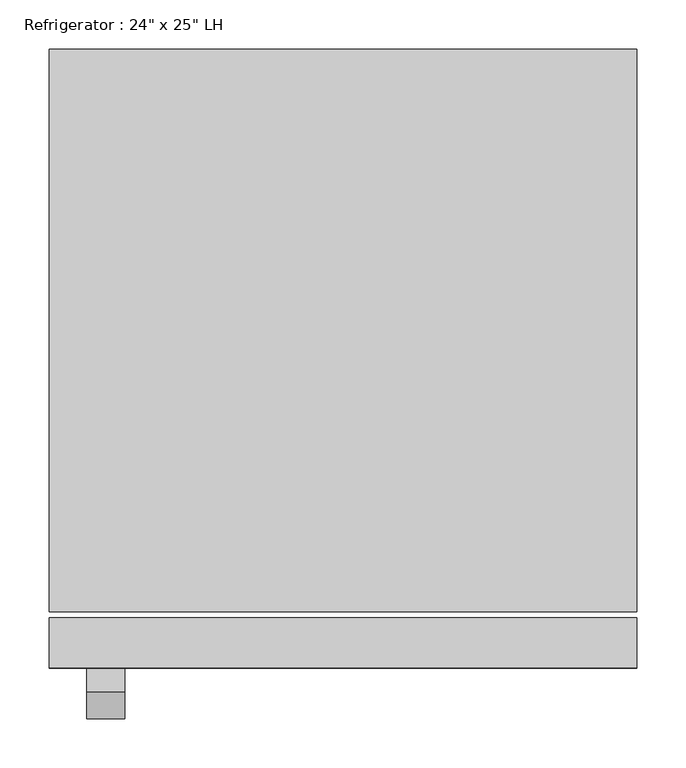
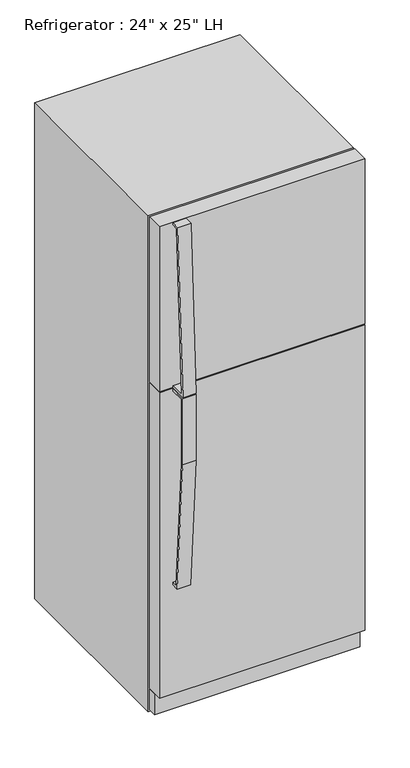
"""IFC4 building model written with IfcOpenShell, lengths in millimetres: proxy geometry."""

from ifc_helpers import new_model, si_unit, frame, origin, origin_with_axes, place, context, project, spatial, polyline, outline, extrude, source, transform, mapped, element, save


def proxy_e2b28e2e(model_context):
    return source(origin(), model_context, "Body", "SweptSolid", [
        extrude(outline(polyline([(-329.0010285, 1008.0625), (-373.4510285, 1008.0625), (-373.4510285, 811.4342469), (-345.9723987, 418.4715334), (-329.0010285, 418.4715334), (-329.0010285, 412.1370017), (-351.8949512, 412.1370017), (-379.8010285, 811.2125), (-379.8010285, 1014.4125), (-329.0010285, 1014.4125), (-329.0010285, 1008.0625)])), frame((-260.35, 0.0, 0.0), z_axis=(1.0, 0.0, 0.0), x_axis=(0.0, 1.0, 0.0)), (0.0, 0.0, 1.0), 38.4332978),
        extrude(outline(polyline([(-353.839413, 1524.0), (-329.7780855, 1524.0), (-329.7780855, 1517.65), (-348.6263449, 1517.65), (-374.5007207, 1023.9375), (-329.7780855, 1023.9375), (-329.7780855, 1017.5875), (-380.3793675, 1017.5875), (-353.839413, 1524.0)])), frame((-260.35, 0.0, 0.0), z_axis=(1.0, 0.0, 0.0), x_axis=(0.0, 1.0, 0.0)), (0.0, 0.0, 1.0), 38.4332978),
        extrude(outline(polyline([(298.45, -278.2010285), (298.45, -303.6010285), (-298.45, -303.6010285), (-298.45, -278.2010285), (298.45, -278.2010285)])), frame((0.0, 0.0, 9.3816357), z_axis=(0.0, 0.0, 1.0), x_axis=(1.0, 0.0, 0.0)), (0.0, 0.0, 1.0), 63.5),
        extrude(outline(polyline([(298.45, -278.2010285), (298.45, -329.0010285), (-298.45, -329.0010285), (-298.45, -278.2010285), (298.45, -278.2010285)])), frame((0.0, 0.0, 76.2), z_axis=(0.0, 0.0, 1.0), x_axis=(1.0, 0.0, 0.0)), (0.0, 0.0, 1.0), 938.2125),
        extrude(outline(polyline([(298.45, -278.2010285), (298.45, -329.0010285), (-298.45, -329.0010285), (-298.45, -278.2010285), (298.45, -278.2010285)])), frame((0.0, 0.0, 1017.5875), z_axis=(0.0, 0.0, 1.0), x_axis=(1.0, 0.0, 0.0)), (0.0, 0.0, 1.0), 506.4125),
        extrude(outline(polyline([(298.45, 299.6489715), (298.45, -271.8510285), (-298.45, -271.8510285), (-298.45, 299.6489715), (298.45, 299.6489715)])), origin_with_axes(), (0.0, 0.0, 1.0), 1524.0),
    ])


if __name__ == "__main__":
    model = new_model("IFC4")
    model_context = context("Model", 3, world=origin())
    ifc_project = project(units=[si_unit("LENGTHUNIT", "METRE", prefix="MILLI")], contexts=[model_context])
    site = spatial("IfcSite", under=ifc_project)
    building = spatial("IfcBuilding", under=site)
    placement = place(None, origin())
    proxy_shape = proxy_e2b28e2e(model_context)
    element("IfcBuildingElementProxy", 1, Name="Refrigerator : 24\" x 25\" LH", ObjectType="Refrigerator : 24\" x 25\" LH", at=placement, inside=building, context=model_context, shape_type="MappedRepresentation", body=[
        mapped(proxy_shape, transform((0.0, 0.0, 0.0), x_axis=(1.0, 0.0, 0.0), y_axis=(0.0, 1.0, 0.0), z_axis=(0.0, 0.0, 1.0))),
    ])
    save(model, "model.ifc")

# Revit data of these elements
# Type "Refrigerator : 24\" x 25\" LH"
#   Label = "REF."
#   Assembly Code = "E1090400"
#   Depth = 2' - 0 3/4"
#   Handle = 0' - 1 1/2"
#   Height = 5' - 0"
#   Rear Clearance = 0' - 2"
#   Top Door Height = 1' - 8"
#   Width = 1' - 11 1/2"
#   Material = Steel, Paint Finish, Ivory, Glossy
#   Default Elevation = 0
# Element 1 (IfcBuildingElementProxy, "Refrigerator : 24\" x 25\" LH")
#   Materials on its faces: "Steel, Paint Finish, Ivory, Glossy", "Steel, Chrome Plated"
# Materials
#   "Steel, Paint Finish, Ivory, Glossy": class "Metal", colour RGB 247 247 239, transparency 0, Description = "Steel, paint finish, ivory, glossy", Cost = 0
#   "Steel, Chrome Plated": class "Metal", colour RGB 17 17 17, transparency 0, Description = "Chromiuim plated steel", Cost = 0
